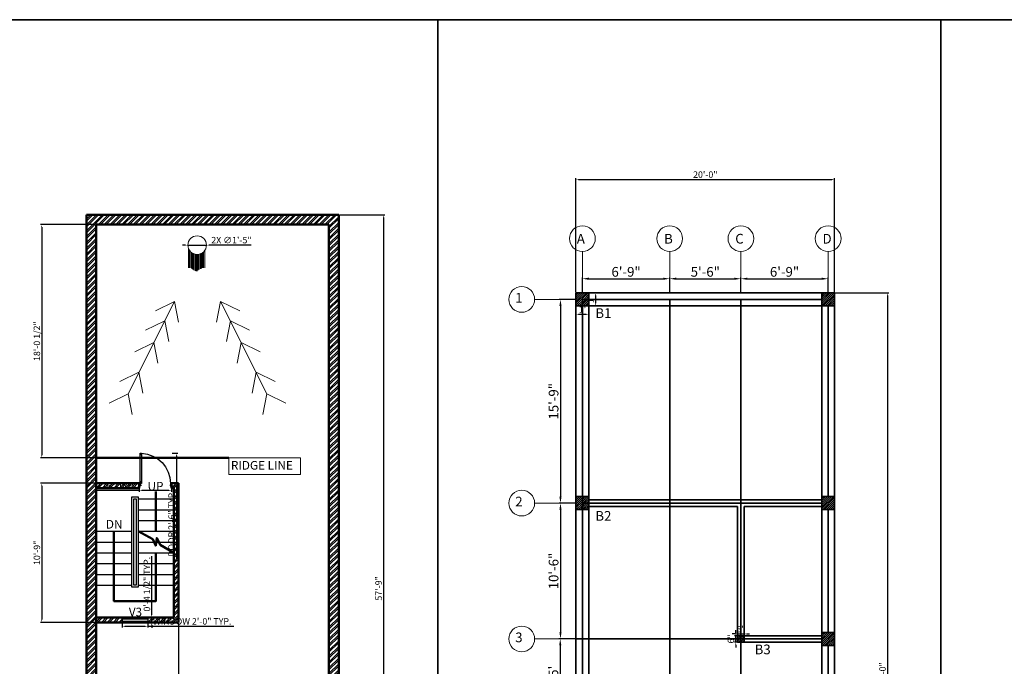
# Model space of a CAD drawing. Units: millimetres. Extents: x 20768 to 23556, y 50760 to 52704.
# Tile 31 of 36: x 21642 to 22556, y 52104 to 52704. Entities that reach past the tile are written whole.
import ezdxf

# ---------------------------------------------------------------- set-up
doc = ezdxf.new("R2010")
doc.units = ezdxf.units.MM
for name, color, linetype, lineweight in [('A-ANNO-TTLB', 7, 'Continuous', 35), ('A-AREA-IDEN', 40, 'Continuous', 18), ('A-DOOR', 3, 'Continuous', 25), ('A-FLOR-STRS', 11, 'Continuous', 25), ('A-GLAZ', 4, 'Continuous', 25), ('A-ROOF', 30, 'Continuous', 18), ('A-WALL', 7, 'Continuous', 50), ('A-WALL-PATT', 8, 'Continuous', 13), ('S-ANNO-DIMS', 2, 'Continuous', 18), ('S-ANNO-TEXT', 6, 'Continuous', 18), ('S-BEAM', 3, 'Continuous', 35), ('S-COLS', 20, 'Continuous', 35), ('S-COLS-PATT', 8, 'Continuous', 13), ('S-GRID', 1, 'Continuous', 18)]:
    doc.layers.add(name, color=color, linetype=linetype, lineweight=lineweight)
doc.styles.get("Standard").update_dxf_attribs({"font": 'arial.ttf'})
doc.dimstyles.new('ISO-25', dxfattribs={"dimtxt": 6, "dimasz": 2.5, "dimexe": 1.25, "dimexo": 0.625, "dimtad": 1, "dimdec": 0, "dimlunit": 3, "dimtxsty": 'Standard', "dimcen": 2.5, "dimadec": 0, "dimazin": 0, "dimtfac": 1, "dimtdec": 0, "dimtmove": 0, "dimatfit": 3, "dimfxl": 1, "dimarcsym": 0})
pattern_1 = [(45, (102.9326, 0), (-0.898025612, 0.898025612), [])]

# ---------------------------------------------------------------- blocks, each defined once
blk = doc.blocks.new('Puerta 01')
for p, q in [((-0.775, -0.026), (-0.737, -0.058)), ((-0.775, -0.058), (-0.737, -0.026)), ((-0.737, -0.058), (-0.737, -0.026)), ((-0.028, -0.058), (-0.066, -0.026)), ((-0.028, -0.026), (-0.066, -0.058)), ((-0.066, -0.058), (-0.066, -0.026))]:
    blk.add_line(p, q)
for points in [[(-0.028, 0), (-0.028, -0.026), (0.004, -0.026), (0.004, -0.036), (0.028, -0.036), (0.028, 0)], [(-0.028, -0.026), (-0.775, -0.026), (-0.775, -0.058), (-0.028, -0.058)], [(0.004, -0.774), (0.004, -0.764), (0.028, -0.764), (0.028, -0.8), (-0.028, -0.8), (-0.028, -0.774)]]:
    blk.add_lwpolyline(points, close=True)
blk.add_arc((-0.028, -0.026), 0.747, 182.4545, 270)
blk = doc.blocks.new('*D32')
at = {"layer": 'Defpoints', "color": 0, "transparency": 16777216}
for p in [(22245.2, 52463.68), (22164.2, 52450.51), (22245.2, 52450.51)]:
    blk.add_point(p, dxfattribs=at)
at = {"layer": 'S-ANNO-DIMS', "color": 0, "lineweight": -2, "transparency": 16777216}
for p, q in [((22164.2, 52451.13), (22164.2, 52464.93)), ((22170.2, 52463.68), (22239.2, 52463.68)), ((22245.2, 52451.13), (22245.2, 52464.93))]:
    blk.add_line(p, q, dxfattribs=at)
at = {"layer": 'S-ANNO-DIMS', "color": 0, "transparency": 16777216}
for points in [[(22170.2, 52464.68), (22170.2, 52462.68), (22164.2, 52463.68)], [(22239.2, 52464.68), (22239.2, 52462.68), (22245.2, 52463.68)]]:
    blk.add_solid(points, dxfattribs=at)
at = {"layer": 'S-ANNO-DIMS', "color": 0, "transparency": 16777216, "insert": (22204.7, 52468.9), "char_height": 9, "attachment_point": 5}
blk.add_mtext('6\'-9"', dxfattribs=at)
blk = doc.blocks.new('*D33')
at = {"layer": 'Defpoints', "color": 0, "transparency": 16777216}
for p in [(22311.2, 52463.68), (22245.2, 52450.51), (22311.2, 52450.51)]:
    blk.add_point(p, dxfattribs=at)
at = {"layer": 'S-ANNO-DIMS', "color": 0, "lineweight": -2, "transparency": 16777216}
for p, q in [((22245.2, 52451.13), (22245.2, 52464.93)), ((22251.2, 52463.68), (22305.2, 52463.68)), ((22311.2, 52451.13), (22311.2, 52464.93))]:
    blk.add_line(p, q, dxfattribs=at)
at = {"layer": 'S-ANNO-DIMS', "color": 0, "transparency": 16777216}
for points in [[(22251.2, 52464.68), (22251.2, 52462.68), (22245.2, 52463.68)], [(22305.2, 52464.68), (22305.2, 52462.68), (22311.2, 52463.68)]]:
    blk.add_solid(points, dxfattribs=at)
at = {"layer": 'S-ANNO-DIMS', "color": 0, "transparency": 16777216, "insert": (22278.2, 52468.9), "char_height": 9, "attachment_point": 5}
blk.add_mtext('5\'-6"', dxfattribs=at)
blk = doc.blocks.new('*D34')
at = {"layer": 'Defpoints', "color": 0, "transparency": 16777216}
for p in [(22392.2, 52463.68), (22311.2, 52450.51), (22392.2, 52450.51)]:
    blk.add_point(p, dxfattribs=at)
at = {"layer": 'S-ANNO-DIMS', "color": 0, "lineweight": -2, "transparency": 16777216}
for p, q in [((22311.2, 52451.13), (22311.2, 52464.93)), ((22317.2, 52463.68), (22386.2, 52463.68)), ((22392.2, 52451.13), (22392.2, 52464.93))]:
    blk.add_line(p, q, dxfattribs=at)
at = {"layer": 'S-ANNO-DIMS', "color": 0, "transparency": 16777216}
for points in [[(22317.2, 52464.68), (22317.2, 52462.68), (22311.2, 52463.68)], [(22386.2, 52464.68), (22386.2, 52462.68), (22392.2, 52463.68)]]:
    blk.add_solid(points, dxfattribs=at)
at = {"layer": 'S-ANNO-DIMS', "color": 0, "transparency": 16777216, "insert": (22351.7, 52468.9), "char_height": 9, "attachment_point": 5}
blk.add_mtext('6\'-9"', dxfattribs=at)
blk = doc.blocks.new('*D35')
at = {"layer": 'Defpoints', "color": 0, "transparency": 16777216}
for p in [(22158.2, 52444.51), (22143.84, 52255.51), (22158.2, 52255.51)]:
    blk.add_point(p, dxfattribs=at)
at = {"layer": 'S-ANNO-DIMS', "color": 0, "lineweight": -2, "transparency": 16777216}
for p, q in [((22157.58, 52444.51), (22142.59, 52444.51)), ((22143.84, 52438.51), (22143.84, 52261.51)), ((22157.58, 52255.51), (22142.59, 52255.51))]:
    blk.add_line(p, q, dxfattribs=at)
at = {"layer": 'S-ANNO-DIMS', "color": 0, "transparency": 16777216}
for points in [[(22142.84, 52438.51), (22144.84, 52438.51), (22143.84, 52444.51)], [(22142.84, 52261.51), (22144.84, 52261.51), (22143.84, 52255.51)]]:
    blk.add_solid(points, dxfattribs=at)
at = {"layer": 'S-ANNO-DIMS', "color": 0, "transparency": 16777216, "insert": (22138.62, 52350.01), "char_height": 9, "attachment_point": 5, "rotation": 90}
blk.add_mtext('15\'-9"', dxfattribs=at)
blk = doc.blocks.new('*D36')
at = {"layer": 'Defpoints', "color": 0, "transparency": 16777216}
for p in [(22158.2, 52255.51), (22143.84, 52129.51), (22158.2, 52129.51)]:
    blk.add_point(p, dxfattribs=at)
at = {"layer": 'S-ANNO-DIMS', "color": 0, "lineweight": -2, "transparency": 16777216}
for p, q in [((22157.58, 52255.51), (22142.59, 52255.51)), ((22143.84, 52249.51), (22143.84, 52135.51)), ((22157.58, 52129.51), (22142.59, 52129.51))]:
    blk.add_line(p, q, dxfattribs=at)
at = {"layer": 'S-ANNO-DIMS', "color": 0, "transparency": 16777216}
for points in [[(22142.84, 52249.51), (22144.84, 52249.51), (22143.84, 52255.51)], [(22142.84, 52135.51), (22144.84, 52135.51), (22143.84, 52129.51)]]:
    blk.add_solid(points, dxfattribs=at)
at = {"layer": 'S-ANNO-DIMS', "color": 0, "transparency": 16777216, "insert": (22138.62, 52192.51), "char_height": 9, "attachment_point": 5, "rotation": 90}
blk.add_mtext('10\'-6"', dxfattribs=at)
blk = doc.blocks.new('*D37')
at = {"layer": 'Defpoints', "color": 0, "transparency": 16777216}
for p in [(22158.2, 52129.51), (22143.63, 52069.51), (22158.2, 52069.51)]:
    blk.add_point(p, dxfattribs=at)
at = {"layer": 'S-ANNO-DIMS', "color": 0, "lineweight": -2, "transparency": 16777216}
for p, q in [((22157.58, 52129.51), (22142.38, 52129.51)), ((22143.63, 52123.51), (22143.63, 52075.51)), ((22157.58, 52069.51), (22142.38, 52069.51))]:
    blk.add_line(p, q, dxfattribs=at)
at = {"layer": 'S-ANNO-DIMS', "color": 0, "transparency": 16777216}
for points in [[(22142.63, 52123.51), (22144.63, 52123.51), (22143.63, 52129.51)], [(22142.63, 52075.51), (22144.63, 52075.51), (22143.63, 52069.51)]]:
    blk.add_solid(points, dxfattribs=at)
at = {"layer": 'S-ANNO-DIMS', "color": 0, "transparency": 16777216, "insert": (22138.43, 52099.51), "char_height": 9, "attachment_point": 5, "rotation": 90}
blk.add_mtext("5'", dxfattribs=at)
blk = doc.blocks.new('*D41')
at = {"layer": 'Defpoints', "color": 0, "transparency": 16777216}
for p in [(22158.2, 52438.51), (22170.2, 52438.51), (22170.2, 52430.74)]:
    blk.add_point(p, dxfattribs=at)
at = {"layer": 'S-ANNO-DIMS', "color": 0, "lineweight": -2, "transparency": 16777216}
for p, q in [((22158.2, 52437.88), (22158.2, 52429.49)), ((22170.2, 52437.88), (22170.2, 52429.49)), ((22160.7, 52430.74), (22167.7, 52430.74))]:
    blk.add_line(p, q, dxfattribs=at)
at = {"layer": 'S-ANNO-DIMS', "color": 0, "transparency": 16777216}
for points in [[(22160.7, 52431.16), (22160.7, 52430.32), (22158.2, 52430.74)], [(22167.7, 52431.16), (22167.7, 52430.32), (22170.2, 52430.74)]]:
    blk.add_solid(points, dxfattribs=at)
at = {"layer": 'S-ANNO-DIMS', "color": 0, "transparency": 16777216, "insert": (22164.2, 52434.38), "char_height": 6, "attachment_point": 5}
blk.add_mtext("1'", dxfattribs=at)
blk = doc.blocks.new('*D42')
at = {"layer": 'Defpoints', "color": 0, "transparency": 16777216}
for p in [(22170.2, 52450.51), (22170.2, 52438.51), (22176.18, 52438.51)]:
    blk.add_point(p, dxfattribs=at)
at = {"layer": 'S-ANNO-DIMS', "color": 0, "lineweight": -2, "transparency": 16777216}
for p, q in [((22170.83, 52450.51), (22177.43, 52450.51)), ((22176.18, 52448.01), (22176.18, 52441.01)), ((22170.83, 52438.51), (22177.43, 52438.51))]:
    blk.add_line(p, q, dxfattribs=at)
at = {"layer": 'S-ANNO-DIMS', "color": 0, "transparency": 16777216}
for points in [[(22175.76, 52448.01), (22176.6, 52448.01), (22176.18, 52450.51)], [(22175.76, 52441.01), (22176.6, 52441.01), (22176.18, 52438.51)]]:
    blk.add_solid(points, dxfattribs=at)
at = {"layer": 'S-ANNO-DIMS', "color": 0, "transparency": 16777216, "insert": (22172.54, 52444.51), "char_height": 6, "attachment_point": 5, "rotation": 90}
blk.add_mtext("1'", dxfattribs=at)
blk = doc.blocks.new('*D45')
at = {"layer": 'Defpoints', "color": 0, "transparency": 16777216}
for p in [(22306.46, 52132.51), (22308.2, 52132.51), (22308.2, 52126.51)]:
    blk.add_point(p, dxfattribs=at)
at = {"layer": 'S-ANNO-DIMS', "color": 0, "lineweight": -2, "transparency": 16777216}
for p, q in [((22307.58, 52132.51), (22305.21, 52132.51)), ((22306.46, 52135.01), (22306.46, 52137.51)), ((22306.46, 52126.51), (22306.46, 52132.51)), ((22307.58, 52126.51), (22305.21, 52126.51)), ((22306.46, 52124.01), (22306.46, 52121.51))]:
    blk.add_line(p, q, dxfattribs=at)
at = {"layer": 'S-ANNO-DIMS', "color": 0, "transparency": 16777216}
for points in [[(22306.04, 52135.01), (22306.87, 52135.01), (22306.46, 52132.51)], [(22306.04, 52124.01), (22306.87, 52124.01), (22306.46, 52126.51)]]:
    blk.add_solid(points, dxfattribs=at)
at = {"layer": 'S-ANNO-DIMS', "color": 0, "transparency": 16777216, "insert": (22302.77, 52129.51), "char_height": 6, "attachment_point": 5, "rotation": 90}
blk.add_mtext('6"', dxfattribs=at)
blk = doc.blocks.new('*D46')
at = {"layer": 'Defpoints', "color": 0, "transparency": 16777216}
for p in [(22308.2, 52132.51), (22314.2, 52134.12), (22314.2, 52132.51)]:
    blk.add_point(p, dxfattribs=at)
at = {"layer": 'S-ANNO-DIMS', "color": 0, "lineweight": -2, "transparency": 16777216}
for p, q in [((22305.7, 52134.12), (22303.2, 52134.12)), ((22308.2, 52133.13), (22308.2, 52135.37)), ((22308.2, 52134.12), (22314.2, 52134.12)), ((22314.2, 52133.13), (22314.2, 52135.37)), ((22316.7, 52134.12), (22319.2, 52134.12))]:
    blk.add_line(p, q, dxfattribs=at)
at = {"layer": 'S-ANNO-DIMS', "color": 0, "transparency": 16777216}
for points in [[(22305.7, 52134.53), (22305.7, 52133.7), (22308.2, 52134.12)], [(22316.7, 52134.53), (22316.7, 52133.7), (22314.2, 52134.12)]]:
    blk.add_solid(points, dxfattribs=at)
at = {"layer": 'S-ANNO-DIMS', "color": 0, "transparency": 16777216, "insert": (22311.2, 52137.8), "char_height": 6, "attachment_point": 5}
blk.add_mtext('6"', dxfattribs=at)
blk = doc.blocks.new('GRID-BUBBLE')
blk.add_line((47.87, 11.93), (23.87, 11.93))
blk.add_circle((11.93, 11.93), 11.93)
blk = doc.blocks.new('WIN-PLAN-B')
blk.add_line((0, 4.5), (0, 0))
blk.add_lwpolyline([(0, 4.5), (24, 4.5), (24, 0), (0, 0)], close=True)
blk = doc.blocks.new('*D171')
at = {"layer": 'Defpoints', "color": 0, "transparency": 16777216}
for p in [(21783.07, 52301.74), (21783.07, 52271.65), (21787.58, 52271.65)]:
    blk.add_point(p, dxfattribs=at)
at = {"layer": 'S-ANNO-DIMS', "color": 0, "lineweight": -2, "transparency": 16777216}
for p, q in [((21783.69, 52301.74), (21788.83, 52301.74)), ((21787.58, 52299.24), (21787.58, 52274.15)), ((21783.69, 52271.65), (21788.83, 52271.65)), ((21787.58, 52271.65), (21787.58, 52204.15))]:
    blk.add_line(p, q, dxfattribs=at)
at = {"layer": 'S-ANNO-DIMS', "color": 0, "transparency": 16777216}
for points in [[(21787.17, 52299.24), (21788, 52299.24), (21787.58, 52301.74)], [(21787.17, 52274.15), (21788, 52274.15), (21787.58, 52271.65)]]:
    blk.add_solid(points, dxfattribs=at)
at = {"layer": 'S-ANNO-DIMS', "color": 0, "transparency": 16777216, "insert": (21783.85, 52236.65), "char_height": 6, "attachment_point": 5, "rotation": 90}
blk.add_mtext('DOOR 2\'-6" TYP.', dxfattribs=at)
blk = doc.blocks.new('*D172')
at = {"layer": 'Defpoints', "color": 0, "transparency": 16777216}
for p in [(21753.07, 52271.65), (21783.07, 52271.65), (21753.07, 52267.13)]:
    blk.add_point(p, dxfattribs=at)
at = {"layer": 'S-ANNO-DIMS', "color": 0, "lineweight": -2, "transparency": 16777216}
for p, q in [((21753.07, 52271.02), (21753.07, 52265.88)), ((21783.07, 52271.02), (21783.07, 52265.88)), ((21753.07, 52267.13), (21712.64, 52267.13)), ((21780.57, 52267.13), (21755.57, 52267.13))]:
    blk.add_line(p, q, dxfattribs=at)
at = {"layer": 'S-ANNO-DIMS', "color": 0, "transparency": 16777216}
for points in [[(21755.57, 52267.55), (21755.57, 52266.72), (21753.07, 52267.13)], [(21780.57, 52267.55), (21780.57, 52266.72), (21783.07, 52267.13)]]:
    blk.add_solid(points, dxfattribs=at)
at = {"layer": 'S-ANNO-DIMS', "color": 0, "transparency": 16777216, "insert": (21731.6, 52270.82), "char_height": 6, "attachment_point": 5}
blk.add_mtext('2\'-6" TYP.', dxfattribs=at)
blk = doc.blocks.new('*D177')
at = {"layer": 'Defpoints', "color": 0, "transparency": 16777216}
for p in [(21737.07, 52144.9), (21761.07, 52144.9), (21761.07, 52141.3)]:
    blk.add_point(p, dxfattribs=at)
at = {"layer": 'S-ANNO-DIMS', "color": 0, "lineweight": -2, "transparency": 16777216}
for p, q in [((21737.07, 52144.27), (21737.07, 52140.05)), ((21761.07, 52144.27), (21761.07, 52140.05)), ((21739.57, 52141.3), (21758.57, 52141.3)), ((21761.07, 52141.3), (21840.74, 52141.3))]:
    blk.add_line(p, q, dxfattribs=at)
at = {"layer": 'S-ANNO-DIMS', "color": 0, "transparency": 16777216}
for points in [[(21739.57, 52141.71), (21739.57, 52140.88), (21737.07, 52141.3)], [(21758.57, 52141.71), (21758.57, 52140.88), (21761.07, 52141.3)]]:
    blk.add_solid(points, dxfattribs=at)
at = {"layer": 'S-ANNO-DIMS', "color": 0, "transparency": 16777216, "insert": (21802.16, 52145.03), "char_height": 6, "attachment_point": 5}
blk.add_mtext('WINDOW 2\'-0" TYP.', dxfattribs=at)
blk = doc.blocks.new('*D178')
at = {"layer": 'Defpoints', "color": 0, "transparency": 16777216}
for p in [(21761.07, 52149.4), (21761.07, 52144.9), (21764.67, 52149.4)]:
    blk.add_point(p, dxfattribs=at)
at = {"layer": 'S-ANNO-DIMS', "color": 0, "lineweight": -2, "transparency": 16777216}
for p, q in [((21764.67, 52151.9), (21764.67, 52206.2)), ((21761.69, 52149.4), (21765.92, 52149.4)), ((21761.69, 52144.9), (21765.92, 52144.9)), ((21764.67, 52144.9), (21764.67, 52149.4)), ((21764.67, 52142.4), (21764.67, 52139.9))]:
    blk.add_line(p, q, dxfattribs=at)
at = {"layer": 'S-ANNO-DIMS', "color": 0, "transparency": 16777216}
for points in [[(21764.25, 52151.9), (21765.08, 52151.9), (21764.67, 52149.4)], [(21764.25, 52142.4), (21765.08, 52142.4), (21764.67, 52144.9)]]:
    blk.add_solid(points, dxfattribs=at)
at = {"layer": 'S-ANNO-DIMS', "color": 0, "transparency": 16777216, "insert": (21760.94, 52180.3), "char_height": 6, "attachment_point": 5, "rotation": 90}
blk.add_mtext('0\'-4 1/2" TYP.', dxfattribs=at)
blk = doc.blocks.new('*D218')
at = {"layer": 'Defpoints', "color": 0, "transparency": 16777216}
for p in [(21938.07, 52522.9), (21938.07, 51829.9), (21979.57, 51829.9)]:
    blk.add_point(p, dxfattribs=at)
at = {"layer": 'S-ANNO-DIMS', "color": 0, "lineweight": -2, "transparency": 16777216}
for p, q in [((21938.69, 52522.9), (21980.82, 52522.9)), ((21979.57, 52520.4), (21979.57, 51832.4)), ((21938.69, 51829.9), (21980.82, 51829.9))]:
    blk.add_line(p, q, dxfattribs=at)
at = {"layer": 'S-ANNO-DIMS', "color": 0, "transparency": 16777216}
for points in [[(21979.15, 52520.4), (21979.98, 52520.4), (21979.57, 52522.9)], [(21979.15, 51832.4), (21979.98, 51832.4), (21979.57, 51829.9)]]:
    blk.add_solid(points, dxfattribs=at)
at = {"layer": 'S-ANNO-DIMS', "color": 0, "transparency": 16777216, "insert": (21975.88, 52176.4), "char_height": 6, "attachment_point": 5, "rotation": 90}
blk.add_mtext('57\'-9"', dxfattribs=at)
blk = doc.blocks.new('*D220')
at = {"layer": 'Defpoints', "color": 0, "transparency": 16777216}
for p in [(21713.07, 52513.9), (21662.57, 52297.64), (21713.07, 52297.64)]:
    blk.add_point(p, dxfattribs=at)
at = {"layer": 'S-ANNO-DIMS', "color": 0, "lineweight": -2, "transparency": 16777216}
for p, q in [((21712.44, 52513.9), (21661.32, 52513.9)), ((21662.57, 52511.4), (21662.57, 52300.14)), ((21712.44, 52297.64), (21661.32, 52297.64))]:
    blk.add_line(p, q, dxfattribs=at)
at = {"layer": 'S-ANNO-DIMS', "color": 0, "transparency": 16777216}
for points in [[(21662.15, 52511.4), (21662.98, 52511.4), (21662.57, 52513.9)], [(21662.15, 52300.14), (21662.98, 52300.14), (21662.57, 52297.64)]]:
    blk.add_solid(points, dxfattribs=at)
at = {"layer": 'S-ANNO-DIMS', "color": 0, "transparency": 16777216, "insert": (21658.84, 52405.77), "char_height": 6, "attachment_point": 5, "rotation": 90}
blk.add_mtext('18\'-0 1/2"', dxfattribs=at)
blk = doc.blocks.new('*D221')
at = {"layer": 'Defpoints', "color": 0, "transparency": 16777216}
for p in [(21713.07, 52273.9), (21662.57, 52144.9), (21713.07, 52144.9)]:
    blk.add_point(p, dxfattribs=at)
at = {"layer": 'S-ANNO-DIMS', "color": 0, "lineweight": -2, "transparency": 16777216}
for p, q in [((21712.44, 52273.9), (21661.32, 52273.9)), ((21662.57, 52271.4), (21662.57, 52147.4)), ((21712.44, 52144.9), (21661.32, 52144.9))]:
    blk.add_line(p, q, dxfattribs=at)
at = {"layer": 'S-ANNO-DIMS', "color": 0, "transparency": 16777216}
for points in [[(21662.15, 52271.4), (21662.98, 52271.4), (21662.57, 52273.9)], [(21662.15, 52147.4), (21662.98, 52147.4), (21662.57, 52144.9)]]:
    blk.add_solid(points, dxfattribs=at)
at = {"layer": 'S-ANNO-DIMS', "color": 0, "transparency": 16777216, "insert": (21658.88, 52209.4), "char_height": 6, "attachment_point": 5, "rotation": 90}
blk.add_mtext('10\'-9"', dxfattribs=at)
blk = doc.blocks.new('*D222')
at = {"layer": 'Defpoints', "color": 0, "transparency": 16777216}
for p in [(21713.07, 52144.9), (21789.57, 52144.9), (21789.57, 51788.4)]:
    blk.add_point(p, dxfattribs=at)
at = {"layer": 'S-ANNO-DIMS', "color": 0, "lineweight": -2, "transparency": 16777216}
for p, q in [((21713.07, 52144.27), (21713.07, 51787.15)), ((21789.57, 52144.27), (21789.57, 51787.15)), ((21715.57, 51788.4), (21787.07, 51788.4))]:
    blk.add_line(p, q, dxfattribs=at)
at = {"layer": 'S-ANNO-DIMS', "color": 0, "transparency": 16777216}
for points in [[(21715.57, 51788.81), (21715.57, 51787.98), (21713.07, 51788.4)], [(21787.07, 51788.81), (21787.07, 51787.98), (21789.57, 51788.4)]]:
    blk.add_solid(points, dxfattribs=at)
at = {"layer": 'S-ANNO-DIMS', "color": 0, "transparency": 16777216, "insert": (21751.32, 51792.12), "char_height": 6, "attachment_point": 5}
blk.add_mtext('6\'-4 1/2"', dxfattribs=at)
blk = doc.blocks.new('*D223')
at = {"layer": 'Defpoints', "color": 0, "transparency": 16777216}
for p in [(22398.2, 52555.8), (22158.2, 52450.51), (22398.2, 52450.51)]:
    blk.add_point(p, dxfattribs=at)
at = {"layer": 'S-ANNO-DIMS', "color": 0, "lineweight": -2, "transparency": 16777216}
for p, q in [((22158.2, 52451.13), (22158.2, 52557.05)), ((22160.7, 52555.8), (22395.7, 52555.8)), ((22398.2, 52451.13), (22398.2, 52557.05))]:
    blk.add_line(p, q, dxfattribs=at)
at = {"layer": 'S-ANNO-DIMS', "color": 0, "transparency": 16777216}
for points in [[(22160.7, 52556.22), (22160.7, 52555.38), (22158.2, 52555.8)], [(22395.7, 52556.22), (22395.7, 52555.38), (22398.2, 52555.8)]]:
    blk.add_solid(points, dxfattribs=at)
at = {"layer": 'S-ANNO-DIMS', "color": 0, "transparency": 16777216, "insert": (22278.2, 52559.49), "char_height": 6, "attachment_point": 5}
blk.add_mtext('20\'-0"', dxfattribs=at)
blk = doc.blocks.new('*D224')
at = {"layer": 'Defpoints', "color": 0, "transparency": 16777216}
for p in [(22398.2, 52450.51), (22398.2, 51742.51), (22447.14, 51742.51)]:
    blk.add_point(p, dxfattribs=at)
at = {"layer": 'S-ANNO-DIMS', "color": 0, "lineweight": -2, "transparency": 16777216}
for p, q in [((22398.83, 52450.51), (22448.39, 52450.51)), ((22447.14, 52448.01), (22447.14, 51745.01)), ((22398.83, 51742.51), (22448.39, 51742.51))]:
    blk.add_line(p, q, dxfattribs=at)
at = {"layer": 'S-ANNO-DIMS', "color": 0, "transparency": 16777216}
for points in [[(22446.72, 52448.01), (22447.56, 52448.01), (22447.14, 52450.51)], [(22446.72, 51745.01), (22447.56, 51745.01), (22447.14, 51742.51)]]:
    blk.add_solid(points, dxfattribs=at)
at = {"layer": 'S-ANNO-DIMS', "color": 0, "transparency": 16777216, "insert": (22443.45, 52096.51), "char_height": 6, "attachment_point": 5, "rotation": 90}
blk.add_mtext('59\'-0"', dxfattribs=at)
blk = doc.blocks.new('*D237')
at = {"layer": 'Defpoints', "color": 0, "transparency": 16777216}
for p in [(21798.19, 52494.85), (21815.37, 52494.84)]:
    blk.add_point(p, dxfattribs=at)
at = {"layer": 'S-ANNO-DIMS', "color": 0, "lineweight": -2, "transparency": 16777216}
for p, q in [((21795.69, 52494.85), (21793.19, 52494.85)), ((21798.19, 52494.85), (21815.37, 52494.84)), ((21856.77, 52494.84), (21817.87, 52494.84))]:
    blk.add_line(p, q, dxfattribs=at)
at = {"layer": 'S-ANNO-DIMS', "color": 0, "transparency": 16777216}
for points in [[(21795.69, 52495.26), (21795.69, 52494.43), (21798.19, 52494.85)], [(21817.87, 52495.26), (21817.87, 52494.43), (21815.37, 52494.84)]]:
    blk.add_solid(points, dxfattribs=at)
at = {"layer": 'S-ANNO-DIMS', "color": 0, "transparency": 16777216, "insert": (21838.57, 52498.7), "char_height": 6, "attachment_point": 5, "rotation": 359.99871}
blk.add_mtext('2X ∅1\'-5"', dxfattribs=at)

msp = doc.modelspace()

# ---------------------------------------------------------------- hatches: boundary and pattern name
at = {"layer": 'A-WALL-PATT'}
h = msp.add_hatch(dxfattribs=at)
h.set_pattern_fill('ANSI32', color=256, scale=0.4)
h.paths.add_polyline_path([(21713.07, 52513.9), (21929.07, 52513.9), (21929.07, 51834.4), (21713.07, 51834.4), (21713.07, 51829.9), (21938.07, 51829.9), (21938.07, 52522.9), (21704.07, 52522.9), (21704.07, 51834.4), (21713.07, 51834.4)])
h = msp.add_hatch(dxfattribs=at)
h.set_pattern_fill('ANSI32', color=256, scale=0.4)
h.paths.add_polyline_path([(21753.07, 52273.9), (21713.07, 52273.9), (21713.07, 52269.4), (21753.07, 52269.4)], flags=17)
h = msp.add_hatch(dxfattribs=at)
h.set_pattern_fill('ANSI32', color=256, scale=0.4)
h.paths.add_polyline_path([(21789.57, 52273.9), (21783.07, 52273.9), (21783.07, 52269.4), (21785.07, 52269.4), (21785.07, 52149.4), (21761.07, 52149.4), (21761.07, 52144.9), (21789.57, 52144.9)], flags=17)
h = msp.add_hatch(dxfattribs=at)
h.set_pattern_fill('ANSI32', color=256, scale=0.4)
h.paths.add_polyline_path([(21737.07, 52149.4), (21713.07, 52149.4), (21713.07, 52144.9), (21737.07, 52144.9)], flags=17)
at = {"layer": 'S-COLS-PATT'}
h = msp.add_hatch(dxfattribs=at)
h.set_pattern_fill('ANSI31', color=256, scale=0.4)
h.set_pattern_definition(pattern_1)
h.paths.add_polyline_path([(22170.2, 52450.51), (22158.2, 52450.51), (22158.2, 52438.51), (22164.2, 52438.51), (22164.2, 52444.51), (22170.2, 52444.51)])
h = msp.add_hatch(dxfattribs=at)
h.set_pattern_fill('ANSI31', color=256, scale=0.4)
h.set_pattern_definition(pattern_1)
h.paths.add_polyline_path([(22170.2, 52444.51), (22164.2, 52444.51), (22164.2, 52438.51), (22170.2, 52438.51)], flags=17)
h = msp.add_hatch(dxfattribs=at)
h.set_pattern_fill('ANSI31', color=256, scale=0.4)
h.set_pattern_definition(pattern_1)
h.paths.add_polyline_path([(22398.2, 52450.51), (22386.2, 52450.51), (22386.2, 52438.51), (22398.2, 52438.51)])
h = msp.add_hatch(dxfattribs=at)
h.set_pattern_fill('ANSI31', color=256, scale=0.4)
h.paths.add_polyline_path([(22164.2, 52261.51), (22158.2, 52261.51), (22158.2, 52249.51), (22164.2, 52249.51)])
h = msp.add_hatch(dxfattribs=at)
h.set_pattern_fill('ANSI31', color=256, scale=0.4)
h.paths.add_polyline_path([(22170.2, 52261.51), (22164.2, 52261.51), (22164.2, 52255.51), (22170.2, 52255.51)])
h = msp.add_hatch(dxfattribs=at)
h.set_pattern_fill('ANSI31', color=256, scale=0.4)
h.set_pattern_definition(pattern_1)
h.paths.add_polyline_path([(22398.2, 52261.51), (22386.2, 52261.51), (22386.2, 52249.51), (22398.2, 52249.51)])
h = msp.add_hatch(dxfattribs=at)
h.set_pattern_fill('ANSI31', color=256, scale=0.4)
h.paths.add_polyline_path([(22170.2, 52255.51), (22164.2, 52255.51), (22164.2, 52249.51), (22170.2, 52249.51)])
h = msp.add_hatch(dxfattribs=at)
h.set_pattern_fill('ANSI31', color=256, scale=0.4)
h.set_pattern_definition(pattern_1)
h.paths.add_polyline_path([(22311.2, 52132.51), (22308.2, 52132.51), (22308.2, 52129.51), (22311.2, 52129.51)])
h = msp.add_hatch(dxfattribs=at)
h.set_pattern_fill('ANSI31', color=256, scale=0.4)
h.set_pattern_definition(pattern_1)
h.paths.add_polyline_path([(22314.2, 52132.51), (22311.2, 52132.51), (22311.2, 52129.51), (22314.2, 52129.51)])
h = msp.add_hatch(dxfattribs=at)
h.set_pattern_fill('ANSI31', color=256, scale=0.4)
h.set_pattern_definition(pattern_1)
h.paths.add_polyline_path([(22398.2, 52135.51), (22386.2, 52135.51), (22386.2, 52123.51), (22398.2, 52123.51)])
h = msp.add_hatch(dxfattribs=at)
h.set_pattern_fill('ANSI31', color=256, scale=0.4)
h.set_pattern_definition(pattern_1)
h.paths.add_polyline_path([(22311.2, 52129.51), (22308.2, 52129.51), (22308.2, 52126.51), (22311.2, 52126.51)], flags=17)
h = msp.add_hatch(dxfattribs=at)
h.set_pattern_fill('ANSI31', color=256, scale=0.4)
h.set_pattern_definition(pattern_1)
h.paths.add_polyline_path([(22314.2, 52129.51), (22311.2, 52129.51), (22311.2, 52126.51), (22314.2, 52126.51)])

# ---------------------------------------------------------------- linework, layer by layer
at = {"layer": 'A-ANNO-TTLB'}
for p, q in [((22029.91, 52703.98), (22029.91, 51623.53)), ((22496.64, 52703.98), (22496.64, 51623.53))]:
    msp.add_line(p, q, dxfattribs=at)
msp.add_lwpolyline([(20768.14, 52703.98), (23555.8, 52703.98), (23555.8, 51623.53), (20768.14, 51623.53)], close=True, dxfattribs=at)
at = {"layer": 'A-FLOR-STRS'}
for p, q in [((21752.07, 52259.4), (21785.07, 52259.4)), ((21752.07, 52249.4), (21785.07, 52249.4)), ((21752.07, 52239.4), (21785.07, 52239.4)), ((21713.07, 52229.4), (21746.07, 52229.4)), ((21752.07, 52229.4), (21785.07, 52229.4)), ((21713.07, 52219.4), (21746.07, 52219.4)), ((21752.07, 52219.4), (21785.07, 52219.4)), ((21713.07, 52209.4), (21746.07, 52209.4)), ((21752.07, 52209.4), (21785.07, 52209.4)), ((21713.07, 52199.4), (21746.07, 52199.4)), ((21752.07, 52199.4), (21785.07, 52199.4)), ((21713.07, 52189.4), (21746.07, 52189.4)), ((21752.07, 52189.4), (21785.07, 52189.4)), ((21713.07, 52179.4), (21746.07, 52179.4)), ((21752.07, 52179.4), (21785.07, 52179.4))]:
    msp.add_line(p, q, dxfattribs=at)
for points in [[(21752.07, 52177.4), (21746.07, 52177.4), (21746.07, 52261.4), (21752.07, 52261.4)], [(21750.07, 52179.4), (21748.07, 52179.4), (21748.07, 52259.4), (21750.07, 52259.4)]]:
    msp.add_lwpolyline(points, close=True, dxfattribs=at)
at = {"layer": 'A-GLAZ'}
for p, q in [((21737.07, 52148.15), (21761.07, 52148.15)), ((21737.07, 52146.15), (21761.07, 52146.15)), ((21761.07, 52149.4), (21761.07, 52144.9))]:
    msp.add_line(p, q, dxfattribs=at)
at = {"layer": 'A-ROOF'}
for p, q in [((21798.78, 52491.72), (21798.78, 52473.92)), ((21799.78, 52489.87), (21799.78, 52473.92)), ((21800.78, 52488.7), (21800.78, 52473.92)), ((21812.78, 52488.7), (21812.78, 52473.92)), ((21813.78, 52489.87), (21813.78, 52473.92)), ((21801.78, 52487.86), (21801.78, 52472.81)), ((21802.78, 52487.24), (21802.78, 52472.39)), ((21803.78, 52486.8), (21803.78, 52471.68)), ((21804.78, 52486.49), (21804.78, 52471)), ((21805.78, 52486.26), (21805.78, 52470.71)), ((21806.78, 52486.26), (21806.78, 52470.75)), ((21807.78, 52486.26), (21807.78, 52471.58)), ((21808.78, 52486.49), (21808.78, 52472.1)), ((21809.78, 52486.8), (21809.78, 52472.94)), ((21810.78, 52487.24), (21810.78, 52473.07)), ((21811.78, 52487.86), (21811.78, 52473.92)), ((21742.75, 52356.89), (21785.65, 52442.62)), ((21871.48, 52356.89), (21828.58, 52442.62))]:
    msp.add_line(p, q, dxfattribs=at)
for points in [[(21767.99, 52434.04), (21785.65, 52442.62), (21789.38, 52423.34)], [(21846.24, 52434.04), (21828.58, 52442.62), (21824.86, 52423.34)], [(21758.97, 52416.01), (21776.63, 52424.58), (21780.35, 52405.31)], [(21855.27, 52416.01), (21837.61, 52424.58), (21833.88, 52405.31)], [(21748.91, 52395.91), (21766.57, 52404.48), (21770.3, 52385.21)], [(21865.32, 52395.91), (21847.66, 52404.48), (21843.94, 52385.21)], [(21735.09, 52368.29), (21752.75, 52376.86), (21756.47, 52357.59)], [(21879.15, 52368.29), (21861.49, 52376.86), (21857.76, 52357.59)], [(21725.09, 52348.32), (21742.75, 52356.89), (21746.48, 52337.62)], [(21889.14, 52348.32), (21871.48, 52356.89), (21867.75, 52337.62)]]:
    msp.add_lwpolyline(points, dxfattribs=at)
msp.add_lwpolyline([(21836.25, 52297.64), (21902.62, 52297.64), (21902.62, 52281.95), (21836.25, 52281.95)], close=True, dxfattribs=at)
msp.add_circle((21806.78, 52494.85), 8.59, dxfattribs=at)
at = {"layer": 'A-WALL'}
for p, q in [((21704.07, 52522.9), (21704.07, 51829.9)), ((21704.07, 52522.9), (21938.07, 52522.9)), ((21938.07, 52522.9), (21938.07, 51829.9)), ((21713.07, 52513.9), (21713.07, 51829.9)), ((21713.07, 52513.9), (21929.07, 52513.9)), ((21929.07, 52513.9), (21929.07, 51834.4)), ((21713.07, 52297.64), (21836.25, 52297.64)), ((21713.07, 52273.9), (21753.07, 52273.9)), ((21713.07, 52269.4), (21753.07, 52269.4)), ((21753.07, 52273.9), (21753.07, 52269.4)), ((21783.07, 52273.9), (21783.07, 52269.4)), ((21783.07, 52273.9), (21789.57, 52273.9)), ((21783.07, 52269.4), (21785.07, 52269.4)), ((21785.07, 52269.4), (21785.07, 52149.4)), ((21789.57, 52273.9), (21789.57, 52144.9)), ((21768.57, 52266.45), (21768.57, 52229.4)), ((21713.07, 52149.4), (21785.07, 52149.4)), ((21713.07, 52144.9), (21789.57, 52144.9))]:
    msp.add_line(p, q, dxfattribs=at)
for points in [[(21768.57, 52209.4), (21768.57, 52164.58), (21729.57, 52164.58), (21729.57, 52229.4)], [(21785.07, 52209.4), (21772.57, 52216.97), (21769.3, 52223.27), (21768.28, 52216.02), (21765.58, 52222.01), (21752.07, 52229.46)]]:
    msp.add_lwpolyline(points, dxfattribs=at)
at = {"layer": 'S-BEAM'}
for p, q in [((22158.2, 52450.51), (22398.2, 52450.51)), ((22158.2, 52450.51), (22158.2, 51742.51)), ((22164.2, 52444.51), (22164.2, 51742.51)), ((22164.2, 52444.51), (22386.2, 52444.51)), ((22170.2, 52450.51), (22170.2, 51742.51)), ((22245.2, 52444.51), (22245.2, 51748.51)), ((22311.2, 52444.51), (22311.2, 51748.51)), ((22386.2, 52450.51), (22386.2, 51742.51)), ((22398.2, 52450.51), (22398.2, 51742.51)), ((22158.2, 52438.51), (22398.2, 52438.51)), ((22392.2, 52438.51), (22392.2, 52261.51)), ((22164.2, 52255.51), (22386.2, 52255.51)), ((22170.2, 52258.51), (22311.2, 52258.51)), ((22170.2, 52252.51), (22308.2, 52252.51)), ((22308.2, 52252.51), (22308.2, 52126.51)), ((22311.2, 52258.51), (22386.2, 52258.51)), ((22314.2, 52252.51), (22314.2, 52126.51)), ((22314.2, 52252.51), (22386.2, 52252.51)), ((22392.2, 52249.51), (22392.2, 52135.51)), ((22308.2, 52132.51), (22386.2, 52132.51)), ((22158.2, 52129.51), (22386.2, 52129.51)), ((22308.2, 52126.51), (22386.2, 52126.51)), ((22392.2, 52123.51), (22392.2, 51823.51))]:
    msp.add_line(p, q, dxfattribs=at)
at = {"layer": 'S-COLS'}
for points in [[(22158.2, 52450.51), (22170.2, 52450.51), (22170.2, 52438.51), (22158.2, 52438.51)], [(22386.2, 52450.51), (22398.2, 52450.51), (22398.2, 52438.51), (22386.2, 52438.51)], [(22170.2, 52261.51), (22158.2, 52261.51), (22158.2, 52249.51), (22170.2, 52249.51)], [(22386.2, 52261.51), (22398.2, 52261.51), (22398.2, 52249.51), (22386.2, 52249.51)], [(22314.2, 52132.51), (22308.2, 52132.51), (22308.2, 52126.51), (22314.2, 52126.51)], [(22386.2, 52135.51), (22398.2, 52135.51), (22398.2, 52123.51), (22386.2, 52123.51)]]:
    msp.add_lwpolyline(points, close=True, dxfattribs=at)
at = {"layer": 'S-GRID'}
for p, q in [((22164.2, 52464.93), (22164.2, 52488.93)), ((22245.2, 52464.93), (22245.2, 52488.93)), ((22311.2, 52464.93), (22311.2, 52488.93)), ((22392.2, 52464.93), (22392.2, 52488.93))]:
    msp.add_line(p, q, dxfattribs=at)
for centre in [(22164.2, 52500.87), (22245.2, 52500.87), (22311.2, 52500.87), (22392.2, 52500.87)]:
    msp.add_circle(centre, 11.93, dxfattribs=at)

# ---------------------------------------------------------------- block references
at = {"layer": 'A-DOOR', "extrusion": (0, 0, -1), "xscale": 37.50000000000053, "yscale": 37.50000000000053, "zscale": -37.50000000000053, "rotation": 270}
msp.add_blockref('Puerta 01', (-21753.07, 52272.7), dxfattribs=at)
at = {"layer": 'A-GLAZ'}
msp.add_blockref('WIN-PLAN-B', (21737.07, 52144.9), dxfattribs=at)
at = {"layer": 'S-GRID'}
for p in [(22095.97, 52432.57), (22095.97, 52243.57), (22095.97, 52117.57)]:
    msp.add_blockref('GRID-BUBBLE', p, dxfattribs=at)

# ---------------------------------------------------------------- texts
at = {"layer": 'A-AREA-IDEN', "char_height": 8, "attachment_point": 1}
for s, width, insert in [('RIDGE LINE', 67.1357, (21838.12, 52294.59)), (' UP', 27.5349, (21758.3, 52275.21)), (' DN', 27.5349, (21719.65, 52239.92)), (' V3', 27.5349, (21740.92, 52158.49))]:
    msp.add_mtext_dynamic_manual_height_columns(s, width=width, gutter_width=12.5, heights=[0], dxfattribs=dict(at, insert=insert))
at = {"layer": 'S-ANNO-TEXT', "char_height": 9, "attachment_point": 1}
for s, width, insert in [('  A', 27.5349, (22153.48, 52505.28)), ('  B', 27.5349, (22234.48, 52505.28)), ('  C', 27.5349, (22300.48, 52505.28)), ('  D', 27.5349, (22381.48, 52505.28)), ('  1', 27.5349, (22096.36, 52450.48)), ('B1', 18.885, (22176.18, 52436.29)), ('  2', 27.5349, (22096.36, 52261.48)), ('B2', 18.885, (22176.18, 52248.15)), ('  3', 27.5349, (22096.36, 52135.48)), ('B3', 18.885, (22323.98, 52124.29))]:
    msp.add_mtext_dynamic_manual_height_columns(s, width=width, gutter_width=12.5, heights=[0], dxfattribs=dict(at, insert=insert))

# ---------------------------------------------------------------- dimensions: what is measured, and where the dimension line sits
at = {"layer": 'S-ANNO-DIMS'}
for base, p1, p2, override, picture, middle in [((22398.2, 52555.8), (22158.2, 52450.51), (22398.2, 52450.51), {"dimdec": 1, "dimlfac": 1, "dimrnd": 0, "dimzin": 1, "dimdsep": 46, "dimlunit": 4, "dimfrac": 2}, '*D223', (22278.2, 52559.49)), ((22245.2, 52463.68), (22164.2, 52450.51), (22245.2, 52450.51), {"dimtxt": 9, "dimasz": 6, "dimclrd": 0, "dimclre": 0, "dimclrt": 0}, '*D32', (22204.7, 52468.9)), ((22311.2, 52463.68), (22245.2, 52450.51), (22311.2, 52450.51), {"dimtxt": 9, "dimasz": 6, "dimclrd": 0, "dimclre": 0, "dimclrt": 0}, '*D33', (22278.2, 52468.9)), ((22392.2, 52463.68), (22311.2, 52450.51), (22392.2, 52450.51), {"dimtxt": 9, "dimasz": 6, "dimclrd": 0, "dimclre": 0, "dimclrt": 0}, '*D34', (22351.7, 52468.9)), ((22170.2, 52430.74), (22158.2, 52438.51), (22170.2, 52438.51), {"dimclrd": 0, "dimclre": 0, "dimclrt": 0}, '*D41', (22164.2, 52434.38)), ((21789.57, 51788.4), (21713.07, 52144.9), (21789.57, 52144.9), {"dimdec": 1, "dimlfac": 1, "dimrnd": 0, "dimzin": 1, "dimdsep": 46, "dimlunit": 4, "dimfrac": 2}, '*D222', (21751.32, 51792.12))]:
    dim = msp.add_linear_dim(base=base, p1=p1, p2=p2, dimstyle='ISO-25', override=override, dxfattribs=at)
    dim.commit()
    dim.dimension.update_dxf_attribs({"geometry": picture, "text_midpoint": middle})
for base, p1, p2, override, picture, middle in [((21979.57, 51829.9), (21938.07, 52522.9), (21938.07, 51829.9), {"dimdec": 1, "dimlfac": 1, "dimrnd": 0, "dimzin": 1, "dimdsep": 46, "dimlunit": 4, "dimfrac": 2}, '*D218', (21975.88, 52176.4)), ((21662.57, 52297.64), (21713.07, 52513.9), (21713.07, 52297.64), {"dimdec": 1, "dimlfac": 1, "dimrnd": 0, "dimzin": 1, "dimdsep": 46, "dimlunit": 4, "dimfrac": 2}, '*D220', (21658.84, 52405.77)), ((22143.84, 52255.51), (22158.2, 52444.51), (22158.2, 52255.51), {"dimtxt": 9, "dimasz": 6, "dimclrd": 0, "dimclre": 0, "dimclrt": 0}, '*D35', (22138.62, 52350.01)), ((22176.18, 52438.51), (22170.2, 52450.51), (22170.2, 52438.51), {"dimclrd": 0, "dimclre": 0, "dimclrt": 0}, '*D42', (22172.54, 52444.51)), ((22447.14, 51742.51), (22398.2, 52450.51), (22398.2, 51742.51), {"dimdec": 1, "dimlfac": 1, "dimrnd": 0, "dimzin": 1, "dimdsep": 46, "dimlunit": 4, "dimfrac": 2}, '*D224', (22443.45, 52096.51)), ((21662.57, 52144.9), (21713.07, 52273.9), (21713.07, 52144.9), {"dimdec": 1, "dimlfac": 1, "dimrnd": 0, "dimzin": 1, "dimdsep": 46, "dimlunit": 4, "dimfrac": 2}, '*D221', (21658.88, 52209.4)), ((22143.84, 52129.51), (22158.2, 52255.51), (22158.2, 52129.51), {"dimtxt": 9, "dimasz": 6, "dimclrd": 0, "dimclre": 0, "dimclrt": 0}, '*D36', (22138.62, 52192.51)), ((22143.63, 52069.51), (22158.2, 52129.51), (22158.2, 52069.51), {"dimtxt": 9, "dimasz": 6, "dimclrd": 0, "dimclre": 0, "dimclrt": 0}, '*D37', (22138.43, 52099.51))]:
    dim = msp.add_linear_dim(base=base, p1=p1, p2=p2, angle=90, dimstyle='ISO-25', override=override, dxfattribs=at)
    dim.commit()
    dim.dimension.update_dxf_attribs({"geometry": picture, "text_midpoint": middle})
dim = msp.add_diameter_dim_2p(p1=(21798.19, 52494.85), p2=(21815.37, 52494.84), text='2X <>', dimstyle='ISO-25', override={"dimdec": 1, "dimlfac": 1, "dimrnd": 0, "dimzin": 1, "dimdsep": 46, "dimlunit": 4, "dimfrac": 2}, dxfattribs=at)
dim.commit()
dim.dimension.update_dxf_attribs({"geometry": '*D237', "text_midpoint": (21838.57, 52494.84), "dimtype": 163})
for base, p1, p2, angle, text, picture, middle in [((21787.58, 52271.65), (21783.07, 52301.74), (21783.07, 52271.65), 270, 'DOOR <> TYP.', '*D171', (21783.85, 52236.65)), ((21753.07, 52267.13), (21783.07, 52271.65), (21753.07, 52271.65), 180, '<> TYP.', '*D172', (21731.6, 52270.82)), ((21764.67, 52149.4), (21761.07, 52144.9), (21761.07, 52149.4), 90, '<> TYP.', '*D178', (21760.94, 52180.3))]:
    dim = msp.add_linear_dim(base=base, p1=p1, p2=p2, angle=angle, text=text, dimstyle='ISO-25', override={"dimdec": 1, "dimrnd": 0, "dimzin": 1, "dimlunit": 4, "dimfrac": 2}, dxfattribs=at)
    dim.commit()
    dim.dimension.update_dxf_attribs({"geometry": picture, "text_midpoint": middle})
dim = msp.add_linear_dim(base=(21761.07, 52141.3), p1=(21737.07, 52144.9), p2=(21761.07, 52144.9), text='WINDOW <> TYP.', dimstyle='ISO-25', override={"dimdec": 1, "dimrnd": 0, "dimzin": 1, "dimlunit": 4, "dimfrac": 2}, dxfattribs=at)
dim.commit()
dim.dimension.update_dxf_attribs({"geometry": '*D177', "text_midpoint": (21802.16, 52145.03)})
dim = msp.add_linear_dim(base=(22314.2, 52134.12), p1=(22308.2, 52132.51), p2=(22314.2, 52132.51), dimstyle='ISO-25', override={"dimclrd": 0, "dimclre": 0, "dimclrt": 0}, dxfattribs=at)
dim.commit()
dim.dimension.update_dxf_attribs({"geometry": '*D46', "text_midpoint": (22311.2, 52134.12), "dimtype": 160})
dim = msp.add_linear_dim(base=(22306.46, 52132.51), p1=(22308.2, 52126.51), p2=(22308.2, 52132.51), angle=90, dimstyle='ISO-25', override={"dimclrd": 0, "dimclre": 0, "dimclrt": 0}, dxfattribs=at)
dim.commit()
dim.dimension.update_dxf_attribs({"geometry": '*D45', "text_midpoint": (22306.46, 52129.51), "dimtype": 160})

doc.saveas('drawing.dxf')
